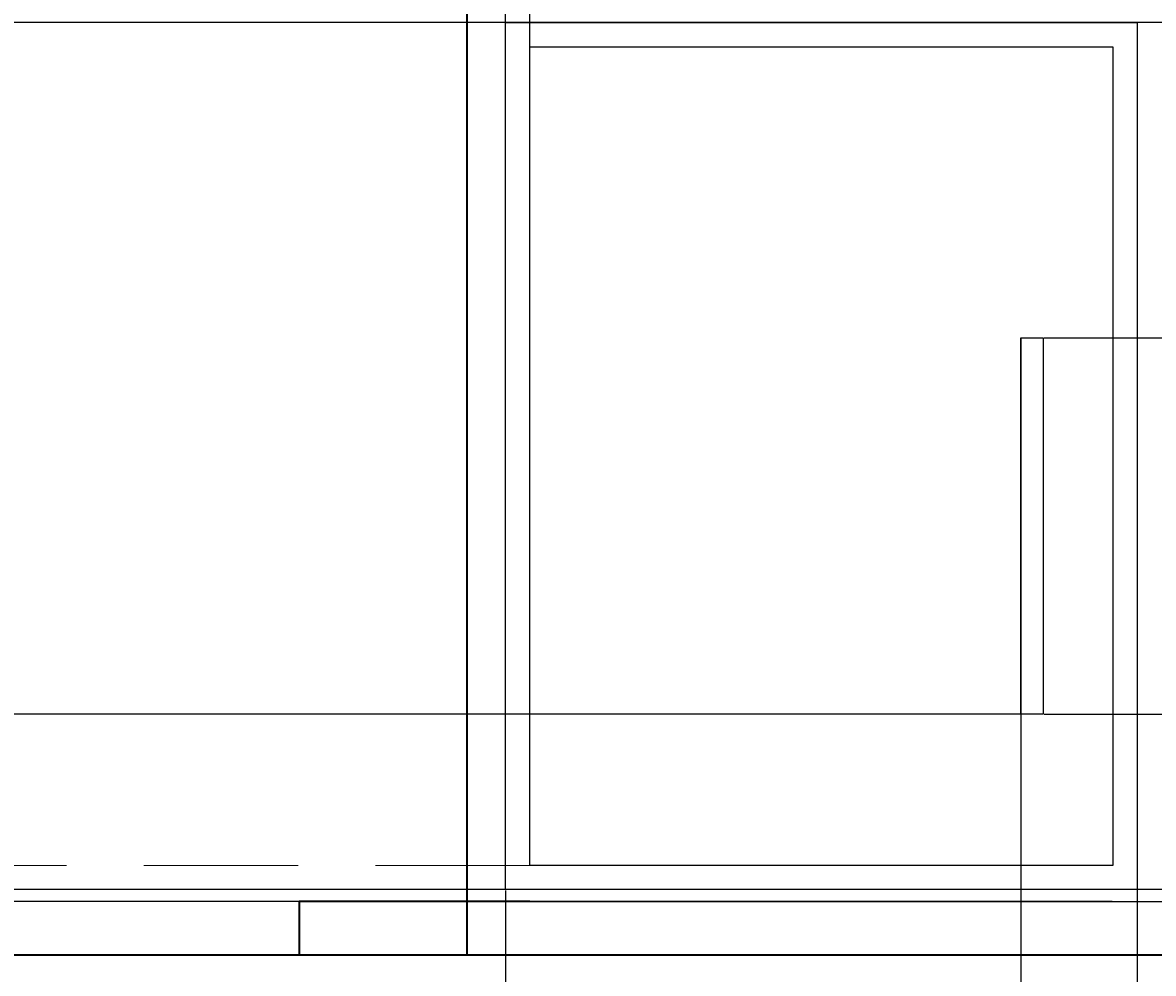
# Model space of a CAD drawing. Units: inches. Extents: x -145 to 510, y 5 to 386.
# Tile 15 of 25: x 182 to 275, y 78 to 157. Entities that reach past the tile are written whole.
import ezdxf

# ---------------------------------------------------------------- set-up
doc = ezdxf.new("R2010")
doc.units = ezdxf.units.IN
doc.header["$MEASUREMENT"] = 0
doc.linetypes.add('DASHED', pattern=[19.05, 12.7, -6.35])
for name, color, linetype, lineweight in [('A-ANNO-DIMS', 2, 'Continuous', 18), ('A-DOOR', 3, 'Continuous', 25), ('A-ELEV', 7, 'Continuous', 35), ('A-ELEV-HIDN', 8, 'DASHED', 18)]:
    doc.layers.add(name, color=color, linetype=linetype, lineweight=lineweight)
doc.styles.get("Standard").update_dxf_attribs({"font": 'arial.ttf'})
doc.dimstyles.get("Standard").update_dxf_attribs({"dimtxt": 0.6875, "dimasz": 0.18, "dimexe": 0.18, "dimexo": 0.0625, "dimgap": 0.09, "dimtad": 0, "dimtih": 1, "dimtoh": 1, "dimdec": 4, "dimzin": 0, "dimdsep": 46, "dimlunit": 4, "dimtxsty": 'Standard', "dimcen": 0.09, "dimadec": 0, "dimazin": 0, "dimtfac": 1, "dimtdec": 4, "dimtofl": 0, "dimtmove": 0, "dimatfit": 3, "dimfxl": 1, "dimtolj": 1, "dimtzin": 0, "dimarcsym": 0})

# ---------------------------------------------------------------- blocks, each defined once
blk = doc.blocks.new('*D9')
at = {"layer": 'A-ANNO-DIMS', "color": 0, "lineweight": -2, "transparency": 16777216}
for p, q in [((159.649, 115.23), (159.649, 5.194)), ((221.529, 85.201), (221.529, 5.194)), ((159.829, 5.374), (189.337, 5.374)), ((221.349, 5.374), (191.842, 5.374))]:
    blk.add_line(p, q, dxfattribs=at)
at = {"layer": 'A-ANNO-DIMS', "color": 0, "transparency": 16777216}
for points in [[(159.829, 5.404), (159.829, 5.344), (159.649, 5.374)], [(221.349, 5.404), (221.349, 5.344), (221.529, 5.374)]]:
    blk.add_solid(points, dxfattribs=at)
at = {"layer": 'Defpoints', "color": 0, "transparency": 16777216}
for p in [(159.649, 115.292), (221.529, 85.264), (221.529, 5.374)]:
    blk.add_point(p, dxfattribs=at)
at = {"layer": 'A-ANNO-DIMS', "color": 0, "transparency": 16777216, "insert": (190.589, 5.374), "char_height": 0.6875, "attachment_point": 5}
blk.add_mtext('\\A1;61.88', dxfattribs=at)
blk = doc.blocks.new('*D10')
at = {"layer": 'A-ANNO-DIMS', "color": 0, "lineweight": -2, "transparency": 16777216}
for p, q in [((221.529, 85.201), (221.529, 5.194)), ((315.554, 85.201), (315.554, 5.194)), ((221.709, 5.374), (267.292, 5.374)), ((315.374, 5.374), (269.792, 5.374))]:
    blk.add_line(p, q, dxfattribs=at)
at = {"layer": 'A-ANNO-DIMS', "color": 0, "transparency": 16777216}
for points in [[(221.709, 5.404), (221.709, 5.344), (221.529, 5.374)], [(315.374, 5.404), (315.374, 5.344), (315.554, 5.374)]]:
    blk.add_solid(points, dxfattribs=at)
at = {"layer": 'Defpoints', "color": 0, "transparency": 16777216}
for p in [(221.529, 85.264), (315.554, 85.264), (315.554, 5.374)]:
    blk.add_point(p, dxfattribs=at)
at = {"layer": 'A-ANNO-DIMS', "color": 0, "transparency": 16777216, "insert": (268.542, 5.374), "char_height": 0.6875, "attachment_point": 5}
blk.add_mtext('\\A1;94.03', dxfattribs=at)
blk = doc.blocks.new('*D19')
at = {"layer": 'A-ANNO-DIMS', "color": 0, "lineweight": -2, "transparency": 16777216}
for p, q in [((478.764, 355.891), (-144.054, 355.891)), ((-143.874, 355.711), (-143.874, 218.332)), ((-143.874, 80.071), (-143.874, 217.45)), ((-114.036, 79.891), (-144.054, 79.891))]:
    blk.add_line(p, q, dxfattribs=at)
at = {"layer": 'A-ANNO-DIMS', "color": 0, "transparency": 16777216}
for points in [[(-143.904, 355.711), (-143.844, 355.711), (-143.874, 355.891)], [(-143.904, 80.071), (-143.844, 80.071), (-143.874, 79.891)]]:
    blk.add_solid(points, dxfattribs=at)
at = {"layer": 'Defpoints', "color": 0, "transparency": 16777216}
for p in [(-143.874, 355.891), (478.826, 355.891), (-113.974, 79.891)]:
    blk.add_point(p, dxfattribs=at)
at = {"layer": 'A-ANNO-DIMS', "color": 0, "transparency": 16777216, "insert": (-143.874, 217.891), "char_height": 0.6875, "attachment_point": 5}
blk.add_mtext('\\A1;276', dxfattribs=at)
blk = doc.blocks.new('*D29')
at = {"layer": 'A-ANNO-DIMS', "color": 0, "lineweight": -2, "transparency": 16777216}
for p, q in [((221.467, 174.992), (-144.054, 174.992)), ((-143.874, 174.812), (-143.874, 130.569)), ((-143.874, 85.444), (-143.874, 129.687)), ((221.467, 85.264), (-144.054, 85.264))]:
    blk.add_line(p, q, dxfattribs=at)
at = {"layer": 'A-ANNO-DIMS', "color": 0, "transparency": 16777216}
for points in [[(-143.904, 174.812), (-143.844, 174.812), (-143.874, 174.992)], [(-143.904, 85.444), (-143.844, 85.444), (-143.874, 85.264)]]:
    blk.add_solid(points, dxfattribs=at)
at = {"layer": 'Defpoints', "color": 0, "transparency": 16777216}
for p in [(-143.874, 174.992), (221.529, 174.992), (221.529, 85.264)]:
    blk.add_point(p, dxfattribs=at)
at = {"layer": 'A-ANNO-DIMS', "color": 0, "transparency": 16777216, "insert": (-143.874, 130.128), "char_height": 0.6875, "attachment_point": 5}
blk.add_mtext('\\A1;89.73', dxfattribs=at)
blk = doc.blocks.new('*D53')
at = {"layer": 'A-ANNO-DIMS', "color": 0, "lineweight": -2, "transparency": 16777216}
for p, q in [((221.529, 85.326), (221.529, 385.971)), ((223.529, 87.326), (223.529, 385.971)), ((221.709, 385.791), (222.211, 385.791)), ((223.349, 385.791), (222.847, 385.791))]:
    blk.add_line(p, q, dxfattribs=at)
at = {"layer": 'A-ANNO-DIMS', "color": 0, "transparency": 16777216}
for points in [[(221.709, 385.821), (221.709, 385.761), (221.529, 385.791)], [(223.349, 385.821), (223.349, 385.761), (223.529, 385.791)]]:
    blk.add_solid(points, dxfattribs=at)
at = {"layer": 'Defpoints', "color": 0, "transparency": 16777216}
for p in [(223.529, 385.791), (223.529, 87.264), (221.529, 85.264)]:
    blk.add_point(p, dxfattribs=at)
at = {"layer": 'A-ANNO-DIMS', "color": 0, "transparency": 16777216, "insert": (222.529, 385.791), "char_height": 0.6875, "attachment_point": 5}
blk.add_mtext('\\A1;2', dxfattribs=at)
blk = doc.blocks.new('*D54')
at = {"layer": 'A-ANNO-DIMS', "color": 0, "lineweight": -2, "transparency": 16777216}
for p, q in [((315.492, 156.609), (-144.054, 156.609)), ((-143.874, 156.429), (-143.874, 121.378)), ((-143.874, 85.444), (-143.874, 120.495)), ((315.492, 85.264), (-144.054, 85.264))]:
    blk.add_line(p, q, dxfattribs=at)
at = {"layer": 'A-ANNO-DIMS', "color": 0, "transparency": 16777216}
for points in [[(-143.904, 156.429), (-143.844, 156.429), (-143.874, 156.609)], [(-143.904, 85.444), (-143.844, 85.444), (-143.874, 85.264)]]:
    blk.add_solid(points, dxfattribs=at)
at = {"layer": 'Defpoints', "color": 0, "transparency": 16777216}
for p in [(-143.874, 156.609), (315.554, 156.609), (315.554, 85.264)]:
    blk.add_point(p, dxfattribs=at)
at = {"layer": 'A-ANNO-DIMS', "color": 0, "transparency": 16777216, "insert": (-143.874, 120.937), "char_height": 0.6875, "attachment_point": 5}
blk.add_mtext('\\A1;71.35', dxfattribs=at)
blk = doc.blocks.new('*D56')
at = {"layer": 'A-ANNO-DIMS', "color": 0, "lineweight": -2, "transparency": 16777216}
for p, q in [((273.491, 156.547), (273.491, 5.194)), ((263.918, 130.608), (263.918, 5.194)), ((264.098, 5.374), (267.458, 5.374)), ((273.311, 5.374), (269.951, 5.374))]:
    blk.add_line(p, q, dxfattribs=at)
at = {"layer": 'A-ANNO-DIMS', "color": 0, "transparency": 16777216}
for points in [[(264.098, 5.404), (264.098, 5.344), (263.918, 5.374)], [(273.311, 5.404), (273.311, 5.344), (273.491, 5.374)]]:
    blk.add_solid(points, dxfattribs=at)
at = {"layer": 'Defpoints', "color": 0, "transparency": 16777216}
for p in [(273.491, 156.609), (263.918, 130.671), (273.491, 5.374)]:
    blk.add_point(p, dxfattribs=at)
at = {"layer": 'A-ANNO-DIMS', "color": 0, "transparency": 16777216, "insert": (268.704, 5.374), "char_height": 0.6875, "attachment_point": 5}
blk.add_mtext('\\A1;9.572', dxfattribs=at)
blk = doc.blocks.new('*D57')
at = {"layer": 'A-ANNO-DIMS', "color": 0, "lineweight": -2, "transparency": 16777216}
for p, q in [((263.856, 99.712), (-144.054, 99.712)), ((-143.874, 99.532), (-143.874, 92.436)), ((-143.874, 84.459), (-143.874, 91.554)), ((271.428, 84.279), (-144.054, 84.279))]:
    blk.add_line(p, q, dxfattribs=at)
at = {"layer": 'A-ANNO-DIMS', "color": 0, "transparency": 16777216}
for points in [[(-143.904, 99.532), (-143.844, 99.532), (-143.874, 99.712)], [(-143.904, 84.459), (-143.844, 84.459), (-143.874, 84.279)]]:
    blk.add_solid(points, dxfattribs=at)
at = {"layer": 'Defpoints', "color": 0, "transparency": 16777216}
for p in [(-143.874, 99.712), (263.918, 99.712), (271.491, 84.279)]:
    blk.add_point(p, dxfattribs=at)
at = {"layer": 'A-ANNO-DIMS', "color": 0, "transparency": 16777216, "insert": (-143.874, 91.995), "char_height": 0.6875, "attachment_point": 5}
blk.add_mtext('\\A1;15.433', dxfattribs=at)
blk = doc.blocks.new('*D58')
at = {"layer": 'A-ANNO-DIMS', "color": 0, "lineweight": -2, "transparency": 16777216}
for p, q in [((265.824, 130.671), (508.906, 130.671)), ((508.726, 130.491), (508.726, 115.632)), ((508.726, 99.892), (508.726, 114.75)), ((265.824, 99.712), (508.906, 99.712))]:
    blk.add_line(p, q, dxfattribs=at)
at = {"layer": 'A-ANNO-DIMS', "color": 0, "transparency": 16777216}
for points in [[(508.696, 130.491), (508.756, 130.491), (508.726, 130.671)], [(508.696, 99.892), (508.756, 99.892), (508.726, 99.712)]]:
    blk.add_solid(points, dxfattribs=at)
at = {"layer": 'Defpoints', "color": 0, "transparency": 16777216}
for p in [(265.761, 130.671), (508.726, 130.671), (265.761, 99.712)]:
    blk.add_point(p, dxfattribs=at)
at = {"layer": 'A-ANNO-DIMS', "color": 0, "transparency": 16777216, "insert": (508.726, 115.191), "char_height": 0.6875, "attachment_point": 5}
blk.add_mtext('\\A1;30.96', dxfattribs=at)

msp = doc.modelspace()

# ---------------------------------------------------------------- linework, layer by layer
at = {"layer": 'A-DOOR'}
for p, q in [((223.5292, 84.2785), (271.4905, 84.2785)), ((271.4905, 84.2785), (278.1416, 84.2785))]:
    msp.add_line(p, q, dxfattribs=at)
for points in [[(221.5292, 156.6093), (273.4905, 156.6093), (273.4905, 85.2638), (221.5292, 85.2638)], [(223.5292, 154.6093), (271.4905, 154.6093), (271.4905, 87.2638), (223.5292, 87.2638)], [(263.9183, 130.6707), (265.7612, 130.6707), (265.7612, 99.7118), (263.9183, 99.7118)]]:
    msp.add_lwpolyline(points, close=True, dxfattribs=at)
at = {"layer": 'A-ELEV'}
for p, q in [((218.3571, 178.0195), (218.3571, 79.8905)), ((223.5292, 84.2785), (204.5552, 84.2785)), ((204.5552, 84.2785), (204.5552, 84.2785)), ((204.5552, 84.2785), (204.5552, 84.2785)), ((204.5552, 84.2785), (204.5552, 79.8905)), ((54.0014, 79.8905), (392.4492, 79.8905))]:
    msp.add_line(p, q, dxfattribs=at)
at = {"layer": 'A-ELEV-HIDN'}
msp.add_line((223.5292, 87.2638), (54.0014, 87.2638), dxfattribs=at)

# ---------------------------------------------------------------- dimensions: what is measured, and where the dimension line sits
at = {"layer": 'A-ANNO-DIMS'}
for base, p1, p2, override, picture, middle in [((223.5292, 385.7905), (221.5292, 85.2638), (223.5292, 87.2638), {"dimdec": 0, "dimlfac": 1, "dimrnd": 0, "dimzin": 0, "dimdsep": 46, "dimlunit": 2}, '*D53', (222.5292, 385.7905)), ((273.4905, 5.3738), (263.9183, 130.6707), (273.4905, 156.6093), {"dimdec": 3, "dimlfac": 1, "dimrnd": 0, "dimzin": 0, "dimdsep": 46, "dimlunit": 2}, '*D56', (268.7044, 5.3738)), ((221.5292, 5.3738), (159.6492, 115.2922), (221.5292, 85.2638), {"dimdec": 2, "dimlfac": 1, "dimrnd": 0, "dimzin": 0, "dimdsep": 46, "dimlunit": 2}, '*D9', (190.5892, 5.3738)), ((315.5545, 5.3738), (221.5292, 85.2638), (315.5545, 85.2638), {"dimdec": 2, "dimlfac": 1, "dimrnd": 0, "dimzin": 0, "dimdsep": 46, "dimlunit": 2}, '*D10', (268.5418, 5.3738))]:
    dim = msp.add_linear_dim(base=base, p1=p1, p2=p2, dimstyle='Standard', override=override, dxfattribs=at)
    dim.commit()
    dim.dimension.update_dxf_attribs({"geometry": picture, "text_midpoint": middle})
for base, p1, p2, override, picture, middle in [((-143.8737, 355.8905), (-113.9737, 79.8905), (478.8263, 355.8905), {"dimdec": 0, "dimlfac": 1, "dimrnd": 0, "dimzin": 0, "dimdsep": 46, "dimlunit": 2}, '*D19', (-143.8737, 217.8905)), ((-143.8737, 174.9923), (221.5292, 85.2638), (221.5292, 174.9923), {"dimdec": 2, "dimlfac": 1, "dimrnd": 0, "dimzin": 0, "dimdsep": 46, "dimlunit": 2}, '*D29', (-143.8737, 130.1281)), ((-143.8737, 156.6093), (315.5545, 85.2638), (315.5545, 156.6093), {"dimdec": 2, "dimlfac": 1, "dimrnd": 0, "dimzin": 0, "dimdsep": 46, "dimlunit": 2}, '*D54', (-143.8737, 120.9365)), ((508.7263, 130.6707), (265.7612, 99.7118), (265.7612, 130.6707), {"dimdec": 2, "dimlfac": 1, "dimrnd": 0, "dimzin": 0, "dimdsep": 46, "dimlunit": 2}, '*D58', (508.7263, 115.1912)), ((-143.8737, 99.7118), (271.4905, 84.2785), (263.9183, 99.7118), {"dimdec": 3, "dimlfac": 1, "dimrnd": 0, "dimzin": 0, "dimdsep": 46, "dimlunit": 2}, '*D57', (-143.8737, 91.9952))]:
    dim = msp.add_linear_dim(base=base, p1=p1, p2=p2, angle=90, dimstyle='Standard', override=override, dxfattribs=at)
    dim.commit()
    dim.dimension.update_dxf_attribs({"geometry": picture, "text_midpoint": middle})

doc.saveas('drawing.dxf')
